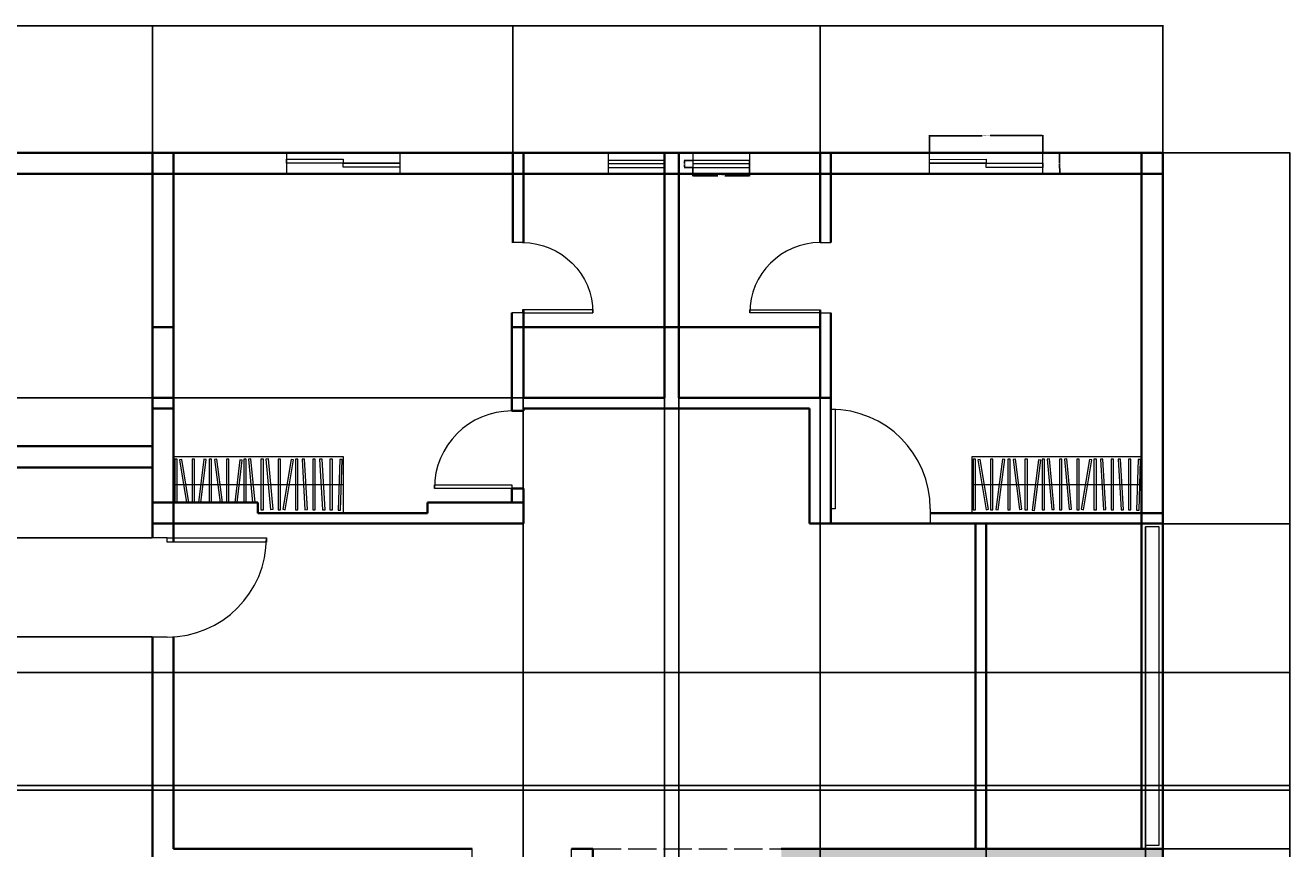
# Model space of a CAD drawing. Units: inches. Extents: x 531915 to 533151, y 849859 to 851471.
# Tile 7 of 7: x 532614 to 533151, y 851121 to 851471. Entities that reach past the tile are written whole.
import ezdxf

# ---------------------------------------------------------------- set-up
doc = ezdxf.new("R2010")
doc.units = ezdxf.units.IN
doc.linetypes.add('ACAD_ISO02W100', pattern=[15, 12, -3])
for name, color, linetype, lineweight in [('A-ANNO-DIMS', 2, 'Continuous', 18), ('A-DOOR', 3, 'Continuous', 18), ('A-FLOR-HRAL', 4, 'Continuous', 20), ('A-FURN', 8, 'Continuous', 13), ('A-GLAZ', 4, 'Continuous', 18), ('A-WALL', 7, 'Continuous', 35), ('A-WALL-OVHD', 7, 'ACAD_ISO02W100', 18), ('A-WALL-PATT', 8, 'Continuous', 13)]:
    doc.layers.add(name, color=color, linetype=linetype, lineweight=lineweight)
doc.styles.get("Standard").update_dxf_attribs({"font": 'arial.ttf'})
doc.dimstyles.get("Standard").update_dxf_attribs({"dimtxt": 0.18, "dimasz": 0.18, "dimexe": 0.18, "dimexo": 0.0625, "dimgap": 0.09, "dimtad": 0, "dimtih": 1, "dimtoh": 1, "dimdec": 4, "dimzin": 0, "dimdsep": 46, "dimtxsty": 'Standard', "dimcen": 0.09, "dimadec": 0, "dimazin": 0, "dimtfac": 1, "dimtdec": 4, "dimtofl": 0, "dimtmove": 0, "dimatfit": 3, "dimfxl": 1, "dimtolj": 1, "dimtzin": 0, "dimarcsym": 0})

# ---------------------------------------------------------------- blocks, each defined once
blk = doc.blocks.new('*U2')
for p, q in [((0, 0), (0, -6)), ((40, 0), (40, -6))]:
    blk.add_line(p, q)
blk.add_lwpolyline([(0, 0), (0, 40), (1.75, 40), (1.75, 0)], close=True)
blk.add_arc((0, 0), 40, 0, 90)
blk = doc.blocks.new('WARDROBE-72')
blk.add_line((12, 0), (12, 72))
for points in [[(24, 0), (24, 72), (0, 72), (0, 0)], [(1.15, 70.47), (1.15, 71.48), (22.64, 71.48), (22.64, 70.47)], [(1.21, 68.56), (1.37, 69.55), (22.58, 66.07), (22.41, 65.07)], [(1.15, 63.15), (1.15, 64.16), (22.64, 64.16), (22.64, 63.15)], [(1.3, 58.13), (1.17, 59.13), (22.48, 61.86), (22.61, 60.86)], [(1.11, 53.59), (1.24, 54.59), (22.54, 51.79), (22.41, 50.79)], [(1.15, 55.83), (1.15, 56.84), (22.64, 56.84), (22.64, 55.83)], [(1.15, 48.51), (1.15, 49.52), (22.64, 49.52), (22.64, 48.51)], [(1.55, 42.84), (1.42, 43.84), (22.76, 46.42), (22.88, 45.42)], [(1.04, 39.13), (1.13, 40.14), (22.52, 38.16), (22.43, 37.15)], [(1.15, 41.19), (1.15, 42.2), (22.64, 42.2), (22.64, 41.19)], [(0.98, 31.76), (1.07, 32.76), (22.47, 30.78), (22.37, 29.78)], [(1.15, 33.87), (1.15, 34.88), (22.64, 34.88), (22.64, 33.87)], [(1.15, 26.55), (1.15, 27.56), (22.64, 27.56), (22.64, 26.55)], [(1.38, 21.1), (1.21, 22.1), (22.4, 25.68), (22.57, 24.68)], [(1.05, 16.46), (1.11, 17.47), (22.56, 16.21), (22.5, 15.2)], [(1.15, 19.23), (1.15, 20.24), (22.64, 20.24), (22.64, 19.23)], [(1.15, 11.91), (1.15, 12.92), (22.64, 12.92), (22.64, 11.91)], [(1.11, 8.97), (1.17, 9.98), (22.62, 8.71), (22.56, 7.7)], [(1.15, 4.59), (1.15, 5.6), (22.64, 5.6), (22.64, 4.59)], [(1.25, 0.42), (1.22, 1.43), (22.7, 2.11), (22.73, 1.1)]]:
    blk.add_lwpolyline(points, close=True)
blk = doc.blocks.new('WARDROBE-72-RECESSED')
blk.add_line((0, 12), (72, 12))
for points in [[(72, 0), (72, 24), (0, 24), (0, 0), (36.16, 0)], [(37.42, 4.5), (39.13, 22.96), (40.14, 22.87), (38.44, 4.5)], [(41.19, 4.5), (41.19, 22.85), (42.2, 22.85), (42.2, 4.5)], [(45.01, 4.5), (42.84, 22.45), (43.84, 22.58), (46.03, 4.5)], [(48.51, 4.5), (48.51, 22.85), (49.52, 22.85), (49.52, 4.5)], [(51.17, 4.5), (53.59, 22.89), (54.59, 22.76), (52.19, 4.5)], [(55.83, 4.5), (55.83, 22.85), (56.84, 22.85), (56.84, 4.5)], [(60.46, 4.5), (58.13, 22.7), (59.13, 22.83), (61.48, 4.5)], [(63.15, 4.5), (63.15, 22.85), (64.16, 22.85), (64.16, 4.5)], [(65.55, 4.5), (68.56, 22.79), (69.55, 22.63), (66.57, 4.5)], [(70.47, 4.5), (70.47, 22.85), (71.48, 22.85), (71.48, 4.5)]]:
    blk.add_lwpolyline(points)
for points in [[(0.42, 22.75), (1.43, 22.78), (2.11, 1.3), (1.1, 1.27)], [(4.59, 22.85), (5.6, 22.85), (5.6, 1.36), (4.59, 1.36)], [(8.97, 22.89), (9.98, 22.83), (8.71, 1.38), (7.7, 1.44)], [(11.91, 22.85), (12.92, 22.85), (12.92, 1.36), (11.91, 1.36)], [(16.46, 22.95), (17.47, 22.89), (16.21, 1.44), (15.2, 1.5)], [(19.23, 22.85), (20.24, 22.85), (20.24, 1.36), (19.23, 1.36)], [(21.1, 22.62), (22.1, 22.79), (25.68, 1.6), (24.68, 1.43)], [(26.55, 22.85), (27.56, 22.85), (27.56, 1.36), (26.55, 1.36)], [(31.76, 23.02), (32.76, 22.93), (30.78, 1.53), (29.78, 1.63)], [(33.87, 22.85), (34.88, 22.85), (34.88, 1.36), (33.87, 1.36)]]:
    blk.add_lwpolyline(points, close=True)
blk = doc.blocks.new('WINDOW-SLIDING-48')
for p, q in [((0, 9), (0, 0)), ((48, 9), (48, 0)), ((0, 4.5), (48, 4.5))]:
    blk.add_line(p, q)
for points in [[(24, 4.5), (48, 4.5), (48, 6.29), (24, 6.29)], [(24, 4.5), (0, 4.5), (0, 2.84), (24, 2.84)]]:
    blk.add_lwpolyline(points, close=True)
blk = doc.blocks.new('WINDOW-VENT-24')
blk.add_line((0, 1.44), (24, 1.44))
blk.add_lwpolyline([(0, 2.89), (24, 2.89), (24, 0), (0, 0)], close=True)
blk = doc.blocks.new('*D19')
at = {"layer": 'A-ANNO-DIMS', "color": 0, "lineweight": -2, "transparency": 16777216}
for p, q in [((532997.8, 851416.94), (532997.79, 851424.26)), ((532997.97, 851424.08), (533020.14, 851424.1)), ((533045.61, 851424.13), (533023.44, 851424.11)), ((533045.8, 851417), (533045.79, 851424.31))]:
    blk.add_line(p, q, dxfattribs=at)
at = {"layer": 'A-ANNO-DIMS', "color": 0, "transparency": 16777216}
for points in [[(532997.97, 851424.11), (532997.97, 851424.05), (532997.79, 851424.08)], [(533045.61, 851424.16), (533045.61, 851424.1), (533045.79, 851424.13)]]:
    blk.add_solid(points, dxfattribs=at)
at = {"layer": 'Defpoints', "color": 0, "transparency": 16777216}
for p in [(533045.79, 851424.13), (532997.8, 851416.88), (533045.8, 851416.93)]:
    blk.add_point(p, dxfattribs=at)
at = {"layer": 'A-ANNO-DIMS', "color": 0, "transparency": 16777216, "insert": (533021.79, 851424.1), "char_height": 0.18, "attachment_point": 5}
blk.add_mtext('\\A1;SLIDING WINDOW 48 TYP.', dxfattribs=at)
blk = doc.blocks.new('*D20')
at = {"layer": 'A-ANNO-DIMS', "color": 0, "lineweight": -2, "transparency": 16777216}
for p, q in [((533045.86, 851416.93), (533053.18, 851416.94)), ((533053, 851416.76), (533053, 851412.63)), ((533053.01, 851408.12), (533053, 851412.26)), ((533045.87, 851407.93), (533053.19, 851407.94))]:
    blk.add_line(p, q, dxfattribs=at)
at = {"layer": 'A-ANNO-DIMS', "color": 0, "transparency": 16777216}
for points in [[(533053.03, 851416.76), (533052.97, 851416.76), (533053, 851416.94)], [(533053.04, 851408.12), (533052.98, 851408.12), (533053.01, 851407.94)]]:
    blk.add_solid(points, dxfattribs=at)
at = {"layer": 'Defpoints', "color": 0, "transparency": 16777216}
for p in [(533045.8, 851416.93), (533045.81, 851407.93), (533053.01, 851407.94)]:
    blk.add_point(p, dxfattribs=at)
at = {"layer": 'A-ANNO-DIMS', "color": 0, "transparency": 16777216, "insert": (533053, 851412.44), "char_height": 0.18, "attachment_point": 5}
blk.add_mtext('\\A1;9 TYP.', dxfattribs=at)
blk = doc.blocks.new('*D21')
at = {"layer": 'A-ANNO-DIMS', "color": 0, "lineweight": -2, "transparency": 16777216}
for p, q in [((532897.3, 851410.6), (532897.3, 851406.88)), ((532897.48, 851407.06), (532907.82, 851407.06)), ((532921.12, 851407.06), (532910.79, 851407.06)), ((532921.3, 851410.6), (532921.3, 851406.88))]:
    blk.add_line(p, q, dxfattribs=at)
at = {"layer": 'A-ANNO-DIMS', "color": 0, "transparency": 16777216}
for points in [[(532897.48, 851407.09), (532897.48, 851407.03), (532897.3, 851407.06)], [(532921.12, 851407.09), (532921.12, 851407.03), (532921.3, 851407.06)]]:
    blk.add_solid(points, dxfattribs=at)
at = {"layer": 'Defpoints', "color": 0, "transparency": 16777216}
for p in [(532897.3, 851410.66), (532897.3, 851407.06), (532921.3, 851410.66)]:
    blk.add_point(p, dxfattribs=at)
at = {"layer": 'A-ANNO-DIMS', "color": 0, "transparency": 16777216, "insert": (532909.3, 851407.06), "char_height": 0.18, "attachment_point": 5}
blk.add_mtext('\\A1;VENT WINDOW 24 TYP.', dxfattribs=at)
blk = doc.blocks.new('*D22')
at = {"layer": 'A-ANNO-DIMS', "color": 0, "lineweight": -2, "transparency": 16777216}
for p, q in [((532897.24, 851413.54), (532893.52, 851413.54)), ((532893.7, 851413.36), (532893.7, 851412.28)), ((532897.24, 851410.66), (532893.52, 851410.66)), ((532893.7, 851410.84), (532893.7, 851411.92))]:
    blk.add_line(p, q, dxfattribs=at)
at = {"layer": 'A-ANNO-DIMS', "color": 0, "transparency": 16777216}
for points in [[(532893.67, 851413.36), (532893.73, 851413.36), (532893.7, 851413.54)], [(532893.67, 851410.84), (532893.73, 851410.84), (532893.7, 851410.66)]]:
    blk.add_solid(points, dxfattribs=at)
at = {"layer": 'Defpoints', "color": 0, "transparency": 16777216}
for p in [(532893.7, 851413.54), (532897.3, 851413.54), (532897.3, 851410.66)]:
    blk.add_point(p, dxfattribs=at)
at = {"layer": 'A-ANNO-DIMS', "color": 0, "transparency": 16777216, "insert": (532893.7, 851412.1), "char_height": 0.18, "attachment_point": 5}
blk.add_mtext('\\A1;3 TYP.', dxfattribs=at)
blk = doc.blocks.new('*D37')
at = {"layer": 'A-ANNO-DIMS', "color": 0, "lineweight": -2, "transparency": 16777216}
for p, q in [((532022.8, 851416.94), (532022.8, 851470.96)), ((532022.98, 851470.78), (532559.45, 851470.78)), ((533096.62, 851470.78), (532560.15, 851470.78)), ((533096.8, 851416.94), (533096.8, 851470.96))]:
    blk.add_line(p, q, dxfattribs=at)
at = {"layer": 'A-ANNO-DIMS', "color": 0, "transparency": 16777216}
for points in [[(532022.98, 851470.81), (532022.98, 851470.75), (532022.8, 851470.78)], [(533096.62, 851470.81), (533096.62, 851470.75), (533096.8, 851470.78)]]:
    blk.add_solid(points, dxfattribs=at)
at = {"layer": 'Defpoints', "color": 0, "transparency": 16777216}
for p in [(533096.8, 851470.78), (532022.8, 851416.87), (533096.8, 851416.87)]:
    blk.add_point(p, dxfattribs=at)
at = {"layer": 'A-ANNO-DIMS', "color": 0, "transparency": 16777216, "insert": (532559.8, 851470.78), "char_height": 0.18, "attachment_point": 5}
blk.add_mtext('\\A1;1074', dxfattribs=at)
blk = doc.blocks.new('*D38')
at = {"layer": 'A-ANNO-DIMS', "color": 0, "lineweight": -2, "transparency": 16777216}
for p, q in [((533096.87, 851416.87), (533150.9, 851416.87)), ((533150.72, 851416.69), (533150.72, 850893.31)), ((533150.72, 850369.55), (533150.72, 850892.94)), ((533056.87, 850369.37), (533150.9, 850369.37))]:
    blk.add_line(p, q, dxfattribs=at)
at = {"layer": 'A-ANNO-DIMS', "color": 0, "transparency": 16777216}
for points in [[(533150.69, 851416.69), (533150.75, 851416.69), (533150.72, 851416.87)], [(533150.69, 850369.55), (533150.75, 850369.55), (533150.72, 850369.37)]]:
    blk.add_solid(points, dxfattribs=at)
at = {"layer": 'Defpoints', "color": 0, "transparency": 16777216}
for p in [(533096.8, 851416.87), (533056.8, 850369.37), (533150.72, 850369.37)]:
    blk.add_point(p, dxfattribs=at)
at = {"layer": 'A-ANNO-DIMS', "color": 0, "transparency": 16777216, "insert": (533150.72, 850893.12), "char_height": 0.18, "attachment_point": 5}
blk.add_mtext('\\A1;1047.5', dxfattribs=at)
blk = doc.blocks.new('*D48')
at = {"layer": 'A-ANNO-DIMS', "color": 0, "lineweight": -2, "transparency": 16777216}
for p, q in [((532667.8, 851416.94), (532667.8, 851470.96)), ((532667.98, 851470.78), (532744.02, 851470.78)), ((532820.62, 851470.78), (532744.59, 851470.78)), ((532820.8, 851416.94), (532820.8, 851470.96))]:
    blk.add_line(p, q, dxfattribs=at)
at = {"layer": 'A-ANNO-DIMS', "color": 0, "transparency": 16777216}
for points in [[(532667.98, 851470.81), (532667.98, 851470.75), (532667.8, 851470.78)], [(532820.62, 851470.81), (532820.62, 851470.75), (532820.8, 851470.78)]]:
    blk.add_solid(points, dxfattribs=at)
at = {"layer": 'Defpoints', "color": 0, "transparency": 16777216}
for p in [(532820.8, 851470.78), (532667.8, 851416.87), (532820.8, 851416.87)]:
    blk.add_point(p, dxfattribs=at)
at = {"layer": 'A-ANNO-DIMS', "color": 0, "transparency": 16777216, "insert": (532744.3, 851470.78), "char_height": 0.18, "attachment_point": 5}
blk.add_mtext('\\A1;153', dxfattribs=at)
blk = doc.blocks.new('*D49')
at = {"layer": 'A-ANNO-DIMS', "color": 0, "lineweight": -2, "transparency": 16777216}
for p, q in [((532825.3, 851312.76), (532825.3, 850315.34)), ((532885.3, 851312.76), (532885.3, 850315.34)), ((532825.48, 850315.52), (532855.09, 850315.52)), ((532885.12, 850315.52), (532855.52, 850315.52))]:
    blk.add_line(p, q, dxfattribs=at)
at = {"layer": 'A-ANNO-DIMS', "color": 0, "transparency": 16777216}
for points in [[(532825.48, 850315.55), (532825.48, 850315.49), (532825.3, 850315.52)], [(532885.12, 850315.55), (532885.12, 850315.49), (532885.3, 850315.52)]]:
    blk.add_solid(points, dxfattribs=at)
at = {"layer": 'Defpoints', "color": 0, "transparency": 16777216}
for p in [(532825.3, 851312.82), (532885.3, 851312.82), (532885.3, 850315.52)]:
    blk.add_point(p, dxfattribs=at)
at = {"layer": 'A-ANNO-DIMS', "color": 0, "transparency": 16777216, "insert": (532855.3, 850315.52), "char_height": 0.18, "attachment_point": 5}
blk.add_mtext('\\A1;60', dxfattribs=at)
blk = doc.blocks.new('*D50')
at = {"layer": 'A-ANNO-DIMS', "color": 0, "lineweight": -2, "transparency": 16777216}
for p, q in [((532891.3, 851312.76), (532891.3, 850315.34)), ((532951.3, 851312.76), (532951.3, 850315.34)), ((532891.48, 850315.52), (532921.09, 850315.52)), ((532951.12, 850315.52), (532921.52, 850315.52))]:
    blk.add_line(p, q, dxfattribs=at)
at = {"layer": 'A-ANNO-DIMS', "color": 0, "transparency": 16777216}
for points in [[(532891.48, 850315.55), (532891.48, 850315.49), (532891.3, 850315.52)], [(532951.12, 850315.55), (532951.12, 850315.49), (532951.3, 850315.52)]]:
    blk.add_solid(points, dxfattribs=at)
at = {"layer": 'Defpoints', "color": 0, "transparency": 16777216}
for p in [(532891.3, 851312.82), (532951.3, 851312.82), (532951.3, 850315.52)]:
    blk.add_point(p, dxfattribs=at)
at = {"layer": 'A-ANNO-DIMS', "color": 0, "transparency": 16777216, "insert": (532921.3, 850315.52), "char_height": 0.18, "attachment_point": 5}
blk.add_mtext('\\A1;60', dxfattribs=at)
blk = doc.blocks.new('*D51')
at = {"layer": 'A-ANNO-DIMS', "color": 0, "lineweight": -2, "transparency": 16777216}
for p, q in [((532951.3, 851416.94), (532951.3, 851470.96)), ((532951.48, 851470.78), (533023.67, 851470.78)), ((533096.62, 851470.78), (533024.44, 851470.78)), ((533096.8, 851416.94), (533096.8, 851470.96))]:
    blk.add_line(p, q, dxfattribs=at)
at = {"layer": 'A-ANNO-DIMS', "color": 0, "transparency": 16777216}
for points in [[(532951.48, 851470.81), (532951.48, 851470.75), (532951.3, 851470.78)], [(533096.62, 851470.81), (533096.62, 851470.75), (533096.8, 851470.78)]]:
    blk.add_solid(points, dxfattribs=at)
at = {"layer": 'Defpoints', "color": 0, "transparency": 16777216}
for p in [(533096.8, 851470.78), (532951.3, 851416.87), (533096.8, 851416.87)]:
    blk.add_point(p, dxfattribs=at)
at = {"layer": 'A-ANNO-DIMS', "color": 0, "transparency": 16777216, "insert": (533024.05, 851470.78), "char_height": 0.18, "attachment_point": 5}
blk.add_mtext('\\A1;145.5', dxfattribs=at)
blk = doc.blocks.new('*D52')
at = {"layer": 'A-ANNO-DIMS', "color": 0, "lineweight": -2, "transparency": 16777216}
for p, q in [((533096.87, 851416.87), (533150.9, 851416.87)), ((533150.72, 851416.69), (533150.72, 851338.31)), ((533150.72, 851259.55), (533150.72, 851337.94)), ((533096.87, 851259.37), (533150.9, 851259.37))]:
    blk.add_line(p, q, dxfattribs=at)
at = {"layer": 'A-ANNO-DIMS', "color": 0, "transparency": 16777216}
for points in [[(533150.69, 851416.69), (533150.75, 851416.69), (533150.72, 851416.87)], [(533150.69, 851259.55), (533150.75, 851259.55), (533150.72, 851259.37)]]:
    blk.add_solid(points, dxfattribs=at)
at = {"layer": 'Defpoints', "color": 0, "transparency": 16777216}
for p in [(533096.8, 851416.87), (533096.8, 851259.37), (533150.72, 851259.37)]:
    blk.add_point(p, dxfattribs=at)
at = {"layer": 'A-ANNO-DIMS', "color": 0, "transparency": 16777216, "insert": (533150.72, 851338.12), "char_height": 0.18, "attachment_point": 5}
blk.add_mtext('\\A1;157.5', dxfattribs=at)
blk = doc.blocks.new('*D53')
at = {"layer": 'A-ANNO-DIMS', "color": 0, "lineweight": -2, "transparency": 16777216}
for p, q in [((533096.87, 851259.37), (533150.9, 851259.37)), ((533150.72, 851259.19), (533150.72, 851190.56)), ((533150.72, 851121.55), (533150.72, 851190.19)), ((533096.87, 851121.37), (533150.9, 851121.37))]:
    blk.add_line(p, q, dxfattribs=at)
at = {"layer": 'A-ANNO-DIMS', "color": 0, "transparency": 16777216}
for points in [[(533150.69, 851259.19), (533150.75, 851259.19), (533150.72, 851259.37)], [(533150.69, 851121.55), (533150.75, 851121.55), (533150.72, 851121.37)]]:
    blk.add_solid(points, dxfattribs=at)
at = {"layer": 'Defpoints', "color": 0, "transparency": 16777216}
for p in [(533096.8, 851259.37), (533096.8, 851121.37), (533150.72, 851121.37)]:
    blk.add_point(p, dxfattribs=at)
at = {"layer": 'A-ANNO-DIMS', "color": 0, "transparency": 16777216, "insert": (533150.72, 851190.37), "char_height": 0.18, "attachment_point": 5}
blk.add_mtext('\\A1;138', dxfattribs=at)
blk = doc.blocks.new('*D54')
at = {"layer": 'A-ANNO-DIMS', "color": 0, "lineweight": -2, "transparency": 16777216}
for p, q in [((533096.87, 851121.37), (533150.9, 851121.37)), ((533150.72, 851121.19), (533150.72, 851034.06)), ((533150.72, 850946.55), (533150.72, 851033.69)), ((533096.87, 850946.37), (533150.9, 850946.37))]:
    blk.add_line(p, q, dxfattribs=at)
at = {"layer": 'A-ANNO-DIMS', "color": 0, "transparency": 16777216}
for points in [[(533150.69, 851121.19), (533150.75, 851121.19), (533150.72, 851121.37)], [(533150.69, 850946.55), (533150.75, 850946.55), (533150.72, 850946.37)]]:
    blk.add_solid(points, dxfattribs=at)
at = {"layer": 'Defpoints', "color": 0, "transparency": 16777216}
for p in [(533096.8, 851121.37), (533096.8, 850946.37), (533150.72, 850946.37)]:
    blk.add_point(p, dxfattribs=at)
at = {"layer": 'A-ANNO-DIMS', "color": 0, "transparency": 16777216, "insert": (533150.72, 851033.87), "char_height": 0.18, "attachment_point": 5}
blk.add_mtext('\\A1;175', dxfattribs=at)
blk = doc.blocks.new('*D58')
at = {"layer": 'A-ANNO-DIMS', "color": 0, "lineweight": -2, "transparency": 16777216}
for p, q in [((533021.8, 851259.31), (533021.8, 850315.34)), ((533089.48, 851257.99), (533089.48, 850315.34)), ((533021.98, 850315.52), (533055.25, 850315.52)), ((533089.3, 850315.52), (533056.04, 850315.52))]:
    blk.add_line(p, q, dxfattribs=at)
at = {"layer": 'A-ANNO-DIMS', "color": 0, "transparency": 16777216}
for points in [[(533021.98, 850315.55), (533021.98, 850315.49), (533021.8, 850315.52)], [(533089.3, 850315.55), (533089.3, 850315.49), (533089.48, 850315.52)]]:
    blk.add_solid(points, dxfattribs=at)
at = {"layer": 'Defpoints', "color": 0, "transparency": 16777216}
for p in [(533021.8, 851259.37), (533089.48, 851258.05), (533089.48, 850315.52)]:
    blk.add_point(p, dxfattribs=at)
at = {"layer": 'A-ANNO-DIMS', "color": 0, "transparency": 16777216, "insert": (533055.64, 850315.52), "char_height": 0.18, "attachment_point": 5}
blk.add_mtext('\\A1;67.67', dxfattribs=at)
blk = doc.blocks.new('*D76')
at = {"layer": 'A-ANNO-DIMS', "color": 0, "lineweight": -2, "transparency": 16777216}
for p, q in [((532820.74, 851416.87), (531968.71, 851416.87)), ((531968.89, 851416.69), (531968.89, 851365.03)), ((531968.89, 851313), (531968.89, 851364.67)), ((532825.24, 851312.82), (531968.71, 851312.82))]:
    blk.add_line(p, q, dxfattribs=at)
at = {"layer": 'A-ANNO-DIMS', "color": 0, "transparency": 16777216}
for points in [[(531968.86, 851416.69), (531968.92, 851416.69), (531968.89, 851416.87)], [(531968.86, 851313), (531968.92, 851313), (531968.89, 851312.82)]]:
    blk.add_solid(points, dxfattribs=at)
at = {"layer": 'Defpoints', "color": 0, "transparency": 16777216}
for p in [(532820.8, 851416.87), (531968.89, 851312.82), (532825.3, 851312.82)]:
    blk.add_point(p, dxfattribs=at)
at = {"layer": 'A-ANNO-DIMS', "color": 0, "transparency": 16777216, "insert": (531968.89, 851364.85), "char_height": 0.18, "attachment_point": 5}
blk.add_mtext('\\A1;104.05', dxfattribs=at)
blk = doc.blocks.new('*D79')
at = {"layer": 'A-ANNO-DIMS', "color": 0, "lineweight": -2, "transparency": 16777216}
for p, q in [((532580.87, 851196.23), (533150.9, 851196.23)), ((533150.72, 851196.05), (533150.72, 851172.42)), ((533150.72, 851148.41), (533150.72, 851172.05)), ((532580.87, 851148.23), (533150.9, 851148.23))]:
    blk.add_line(p, q, dxfattribs=at)
at = {"layer": 'A-ANNO-DIMS', "color": 0, "transparency": 16777216}
for points in [[(533150.69, 851196.05), (533150.75, 851196.05), (533150.72, 851196.23)], [(533150.69, 851148.41), (533150.75, 851148.41), (533150.72, 851148.23)]]:
    blk.add_solid(points, dxfattribs=at)
at = {"layer": 'Defpoints', "color": 0, "transparency": 16777216}
for p in [(532580.8, 851196.23), (532580.8, 851148.23), (533150.72, 851148.23)]:
    blk.add_point(p, dxfattribs=at)
at = {"layer": 'A-ANNO-DIMS', "color": 0, "transparency": 16777216, "insert": (533150.72, 851172.23), "char_height": 0.18, "attachment_point": 5}
blk.add_mtext('\\A1;48', dxfattribs=at)
blk = doc.blocks.new('*D80')
at = {"layer": 'A-ANNO-DIMS', "color": 0, "lineweight": -2, "transparency": 16777216}
for p, q in [((532580.87, 851146.23), (533150.9, 851146.23)), ((533150.72, 851146.05), (533150.72, 851111.42)), ((533150.72, 851076.41), (533150.72, 851111.05)), ((532580.87, 851076.23), (533150.9, 851076.23))]:
    blk.add_line(p, q, dxfattribs=at)
at = {"layer": 'A-ANNO-DIMS', "color": 0, "transparency": 16777216}
for points in [[(533150.69, 851146.05), (533150.75, 851146.05), (533150.72, 851146.23)], [(533150.69, 851076.41), (533150.75, 851076.41), (533150.72, 851076.23)]]:
    blk.add_solid(points, dxfattribs=at)
at = {"layer": 'Defpoints', "color": 0, "transparency": 16777216}
for p in [(532580.8, 851146.23), (532580.8, 851076.23), (533150.72, 851076.23)]:
    blk.add_point(p, dxfattribs=at)
at = {"layer": 'A-ANNO-DIMS', "color": 0, "transparency": 16777216, "insert": (533150.72, 851111.23), "char_height": 0.18, "attachment_point": 5}
blk.add_mtext('\\A1;70', dxfattribs=at)
blk = doc.blocks.new('*D83')
at = {"layer": 'A-ANNO-DIMS', "color": 0, "lineweight": -2, "transparency": 16777216}
for p, q in [((532667.74, 851253.37), (531968.71, 851253.37)), ((531968.89, 851253.19), (531968.89, 851232.55)), ((531968.89, 851211.55), (531968.89, 851232.19)), ((532667.74, 851211.37), (531968.71, 851211.37))]:
    blk.add_line(p, q, dxfattribs=at)
at = {"layer": 'A-ANNO-DIMS', "color": 0, "transparency": 16777216}
for points in [[(531968.86, 851253.19), (531968.92, 851253.19), (531968.89, 851253.37)], [(531968.86, 851211.55), (531968.92, 851211.55), (531968.89, 851211.37)]]:
    blk.add_solid(points, dxfattribs=at)
at = {"layer": 'Defpoints', "color": 0, "transparency": 16777216}
for p in [(531968.89, 851253.37), (532667.8, 851253.37), (532667.8, 851211.37)]:
    blk.add_point(p, dxfattribs=at)
at = {"layer": 'A-ANNO-DIMS', "color": 0, "transparency": 16777216, "insert": (531968.89, 851232.37), "char_height": 0.18, "attachment_point": 5}
blk.add_mtext('\\A1;42', dxfattribs=at)

msp = doc.modelspace()

# ---------------------------------------------------------------- hatches: boundary and pattern name
at = {"layer": 'A-WALL-PATT'}
h = msp.add_hatch(color=256, dxfattribs=at)
h.dxf.hatch_style = 1
h.paths.add_polyline_path([(533096.8048, 851121.374), (532951.8048, 851121.374), (532934.8048, 851121.374), (532934.8048, 851112.374), (533087.8048, 851112.374), (533087.8048, 851106.374), (533096.8048, 851106.374)])

# ---------------------------------------------------------------- linework, layer by layer
at = {"layer": 'A-FLOR-HRAL'}
msp.add_lwpolyline([(533095.2002, 851258.0527), (533089.477, 851258.0527), (533089.477, 851122.9414), (533095.2002, 851122.9414)], close=True, dxfattribs=at)
at = {"layer": 'A-GLAZ'}
for p, q in [((532861.3048, 851416.874), (532861.3048, 851407.874)), ((532897.3048, 851416.874), (532897.3048, 851407.874)), ((532921.3048, 851416.874), (532921.3048, 851407.874))]:
    msp.add_line(p, q, dxfattribs=at)
at = {"layer": 'A-WALL'}
for p, q in [((532022.8048, 851416.874), (533096.8048, 851416.874)), ((533096.8048, 851416.874), (532022.8048, 851416.874)), ((532451.8048, 851416.874), (532667.8048, 851416.874)), ((532667.8048, 851416.874), (532451.8048, 851416.874)), ((532667.8048, 851416.874), (532667.8048, 851253.374)), ((532667.8048, 851416.874), (532667.8048, 851253.374)), ((532676.8048, 851416.874), (532676.8048, 851251.5304)), ((532676.8048, 851416.874), (532676.8048, 851251.5304)), ((532820.8048, 851416.874), (532676.8048, 851416.874)), ((532820.8048, 851416.874), (532820.8048, 851378.7079)), ((532825.3048, 851416.874), (532825.3048, 851378.706)), ((532885.3048, 851416.874), (532885.3048, 851312.8243)), ((532891.3048, 851416.874), (532891.3048, 851312.8243)), ((532951.3048, 851416.874), (532951.3048, 851378.7079)), ((532955.8048, 851416.874), (532955.8048, 851378.7079)), ((533087.8048, 851416.874), (532955.8048, 851416.874)), ((533087.8048, 851416.874), (533087.8048, 851121.374)), ((533096.8048, 851416.874), (533096.8048, 850946.374)), ((533096.8048, 851416.874), (533096.8048, 850946.374)), ((532022.8048, 851407.874), (533096.8048, 851407.874)), ((533096.8048, 851407.874), (532022.8048, 851407.874)), ((532820.4846, 851348.8243), (532820.4846, 851307.227)), ((532825.3048, 851350.1317), (532825.3048, 851312.8243)), ((532951.3048, 851350.1317), (532951.3048, 851312.8243)), ((532955.8048, 851348.8243), (532955.8048, 851259.374)), ((532676.8048, 851342.8243), (532667.8048, 851342.8243)), ((532951.3048, 851342.8243), (532820.4846, 851342.8243)), ((532676.8048, 851312.8243), (532667.8048, 851312.8243)), ((532885.3048, 851312.8243), (532825.3048, 851312.8243)), ((532955.8048, 851312.8243), (532891.3048, 851312.8243)), ((532676.8048, 851308.3243), (532667.8048, 851308.3243)), ((532820.4846, 851307.2354), (532825.3048, 851307.2354)), ((532825.3048, 851308.3243), (532825.3048, 851307.227)), ((532946.8048, 851308.3243), (532825.3048, 851308.3243)), ((532946.8048, 851308.3243), (532946.8048, 851259.374)), ((532451.8048, 851292.2344), (532667.8048, 851292.2344)), ((532451.8048, 851283.2344), (532667.8048, 851283.2344)), ((532820.4846, 851274.374), (532820.4846, 851268.374)), ((532820.4846, 851274.374), (532825.3048, 851274.374)), ((532825.3048, 851274.374), (532825.3048, 851259.374)), ((532712.6447, 851268.374), (532667.8048, 851268.374)), ((532712.6447, 851268.374), (532676.8048, 851268.374)), ((532712.6447, 851268.374), (532676.8048, 851268.374)), ((532712.6447, 851268.374), (532712.6447, 851263.874)), ((532820.4846, 851268.374), (532784.6447, 851268.374)), ((532820.4846, 851268.374), (532784.6447, 851268.374)), ((532820.4846, 851268.374), (532784.6447, 851268.374)), ((532784.6447, 851268.374), (532784.6447, 851263.874)), ((532820.4846, 851268.374), (532825.3048, 851268.374)), ((532784.6447, 851263.874), (532712.6447, 851263.874)), ((533096.8048, 851263.874), (532998.0565, 851263.874)), ((532825.3048, 851259.374), (532667.8048, 851259.374)), ((532955.8048, 851259.374), (532946.8048, 851259.374)), ((532955.8048, 851259.374), (532991.8048, 851259.374)), ((532991.8048, 851259.374), (532997.8048, 851259.374)), ((533096.8048, 851259.374), (532995.8048, 851259.374)), ((533017.3048, 851259.374), (533017.3048, 851121.374)), ((533021.8048, 851259.374), (533021.8048, 851121.374)), ((532667.8048, 851211.374), (532667.8048, 850946.374)), ((532667.8048, 851211.374), (532667.8048, 850369.374)), ((532676.8048, 851211.374), (532676.8048, 851121.374)), ((532676.8048, 851211.374), (532676.8048, 851121.374)), ((532676.8048, 851121.374), (532803.553, 851121.374)), ((532854.8048, 851121.374), (532845.8048, 851121.374)), ((532854.8048, 851121.374), (532854.8048, 851067.874)), ((532934.8048, 851121.374), (533078.8048, 851121.374)), ((533096.8048, 851121.374), (532951.8048, 851121.374))]:
    msp.add_line(p, q, dxfattribs=at)
at = {"layer": 'A-WALL-OVHD'}
msp.add_line((532854.8048, 851121.374), (532934.8048, 851121.374), dxfattribs=at)

# ---------------------------------------------------------------- block references
at = {"layer": 'A-DOOR'}
for p, xscale, yscale, zscale, rotation in [((532824.9671, 851348.8243), -0.7470890379753774, 0.7470890379753774, 0.7470890379753774, 270), ((532951.3222, 851348.8243), 0.7470890379753774, 0.7470890379753774, 0.7470890379753774, 90.00000000000003), ((532820.3768, 851274.374), 0.8213266256042635, 0.8213266256042635, 0.8213266256042635, 90.00000000000003), ((532674.1257, 851253.374), 1.053488616942954, 1.053488616942954, 1.053488616942954, 270), ((532845.8048, 851115.0362), 1.056294156906435, 1.056294156906435, 1.056294156906435, 180)]:
    msp.add_blockref('*U2', p, dxfattribs=dict(at, xscale=xscale, yscale=yscale, zscale=zscale, rotation=rotation))
at = {"layer": 'A-DOOR', "xscale": 1.056294156906435, "yscale": 1.056294156906435, "zscale": 1.056294156906435}
msp.add_blockref('*U2', (532955.8048, 851265.7117), dxfattribs=at)
at = {"layer": 'A-FURN', "extrusion": (0, 0, -1), "zscale": -1}
msp.add_blockref('WARDROBE-72-RECESSED', (-532748.8048, 851263.874), dxfattribs=at)
at = {"layer": 'A-FURN', "extrusion": (0, 0, -1), "zscale": -1, "rotation": 269.9999999994934}
msp.add_blockref('WARDROBE-72', (-533087.8048, 851287.874), dxfattribs=at)
at = {"layer": 'A-GLAZ', "extrusion": (0, 0, -1), "zscale": -1}
for name, p in [('WINDOW-SLIDING-48', (-532772.8048, 851407.874)), ('WINDOW-VENT-24', (-532885.3048, 851410.6579)), ('WINDOW-VENT-24', (-532921.3048, 851410.6579))]:
    msp.add_blockref(name, p, dxfattribs=at)
at = {"layer": 'A-GLAZ', "extrusion": (0, 0, -1), "zscale": -1, "rotation": 179.9286429434092}
msp.add_blockref('WINDOW-SLIDING-48', (-532997.7992, 851416.875), dxfattribs=at)

# ---------------------------------------------------------------- dimensions: what is measured, and where the dimension line sits
at = {"layer": 'A-ANNO-DIMS'}
for base, p1, p2, override, picture, middle in [((533096.8048, 851470.7848), (532022.8048, 851416.874), (533096.8048, 851416.874), {"dimdec": 0, "dimlfac": 1, "dimrnd": 0, "dimzin": 0, "dimdsep": 46, "dimlunit": 2}, '*D37', (532559.8048, 851470.7848)), ((532820.8048, 851470.7848), (532667.8048, 851416.874), (532820.8048, 851416.874), {"dimdec": 0, "dimlfac": 1, "dimrnd": 0, "dimzin": 0, "dimdsep": 46, "dimlunit": 2}, '*D48', (532744.3048, 851470.7848)), ((533096.8048, 851470.7848), (532951.3048, 851416.874), (533096.8048, 851416.874), {"dimdec": 1, "dimlfac": 1, "dimrnd": 0, "dimzin": 0, "dimdsep": 46, "dimlunit": 2}, '*D51', (533024.0548, 851470.7848)), ((532885.3048, 850315.524), (532825.3048, 851312.8243), (532885.3048, 851312.8243), {"dimdec": 0, "dimlfac": 1, "dimrnd": 0, "dimzin": 0, "dimdsep": 46, "dimlunit": 2}, '*D49', (532855.3048, 850315.524)), ((532951.3048, 850315.524), (532891.3048, 851312.8243), (532951.3048, 851312.8243), {"dimdec": 0, "dimlfac": 1, "dimrnd": 0, "dimzin": 0, "dimdsep": 46, "dimlunit": 2}, '*D50', (532921.3048, 850315.524)), ((533089.477, 850315.524), (533021.8048, 851259.374), (533089.477, 851258.0527), {"dimdec": 2, "dimlfac": 1, "dimrnd": 0, "dimzin": 0, "dimdsep": 46, "dimlunit": 2}, '*D58', (533055.6409, 850315.524))]:
    dim = msp.add_linear_dim(base=base, p1=p1, p2=p2, dimstyle='Standard', override=override, dxfattribs=at)
    dim.commit()
    dim.dimension.update_dxf_attribs({"geometry": picture, "text_midpoint": middle})
for base, p1, p2, angle, text, picture, middle in [((533045.7902, 851424.1348), (532997.7992, 851416.875), (533045.7991, 851416.9348), 0.071357, 'SLIDING WINDOW <> TYP.', '*D19', (533021.7902, 851424.1049)), ((532893.7048, 851413.5444), (532897.3048, 851410.6579), (532897.3048, 851413.5444), 90, '<> TYP.', '*D22', (532893.7048, 851412.1011)), ((533053.0103, 851407.9438), (533045.7991, 851416.9348), (533045.8103, 851407.9348), 270.071357, '<> TYP.', '*D20', (533053.0047, 851412.4438)), ((532897.3048, 851407.0579), (532921.3048, 851410.6579), (532897.3048, 851410.6579), 180, 'VENT WINDOW <> TYP.', '*D21', (532909.3048, 851407.0579))]:
    dim = msp.add_linear_dim(base=base, p1=p1, p2=p2, angle=angle, text=text, dimstyle='Standard', override={"dimdec": 0, "dimlfac": 1, "dimrnd": 0, "dimzin": 0, "dimdsep": 46, "dimlunit": 2}, dxfattribs=at)
    dim.commit()
    dim.dimension.update_dxf_attribs({"geometry": picture, "text_midpoint": middle})
for base, p1, p2, override, picture, middle in [((531968.8939, 851312.8243), (532820.8048, 851416.874), (532825.3048, 851312.8243), {"dimdec": 2, "dimlfac": 1, "dimrnd": 0, "dimzin": 0, "dimdsep": 46, "dimlunit": 2}, '*D76', (531968.8939, 851364.8491)), ((533150.7156, 850369.374), (533096.8048, 851416.874), (533056.8048, 850369.374), {"dimdec": 1, "dimlfac": 1, "dimrnd": 0, "dimzin": 0, "dimdsep": 46, "dimlunit": 2}, '*D38', (533150.7156, 850893.124)), ((533150.7156, 851259.374), (533096.8048, 851416.874), (533096.8048, 851259.374), {"dimdec": 1, "dimlfac": 1, "dimrnd": 0, "dimzin": 0, "dimdsep": 46, "dimlunit": 2}, '*D52', (533150.7156, 851338.124)), ((533150.7156, 851121.374), (533096.8048, 851259.374), (533096.8048, 851121.374), {"dimdec": 0, "dimlfac": 1, "dimrnd": 0, "dimzin": 0, "dimdsep": 46, "dimlunit": 2}, '*D53', (533150.7156, 851190.374)), ((531968.8939, 851253.374), (532667.8048, 851211.374), (532667.8048, 851253.374), {"dimdec": 0, "dimlfac": 1, "dimrnd": 0, "dimzin": 0, "dimdsep": 46, "dimlunit": 2}, '*D83', (531968.8939, 851232.374)), ((533150.7156, 851148.2344), (532580.8048, 851196.2344), (532580.8048, 851148.2344), {"dimdec": 0, "dimlfac": 1, "dimrnd": 0, "dimzin": 0, "dimdsep": 46, "dimlunit": 2}, '*D79', (533150.7156, 851172.2344)), ((533150.7156, 851076.2344), (532580.8048, 851146.2344), (532580.8048, 851076.2344), {"dimdec": 0, "dimlfac": 1, "dimrnd": 0, "dimzin": 0, "dimdsep": 46, "dimlunit": 2}, '*D80', (533150.7156, 851111.2344)), ((533150.7156, 850946.374), (533096.8048, 851121.374), (533096.8048, 850946.374), {"dimdec": 0, "dimlfac": 1, "dimrnd": 0, "dimzin": 0, "dimdsep": 46, "dimlunit": 2}, '*D54', (533150.7156, 851033.874))]:
    dim = msp.add_linear_dim(base=base, p1=p1, p2=p2, angle=90, dimstyle='Standard', override=override, dxfattribs=at)
    dim.commit()
    dim.dimension.update_dxf_attribs({"geometry": picture, "text_midpoint": middle})

doc.saveas('drawing.dxf')
